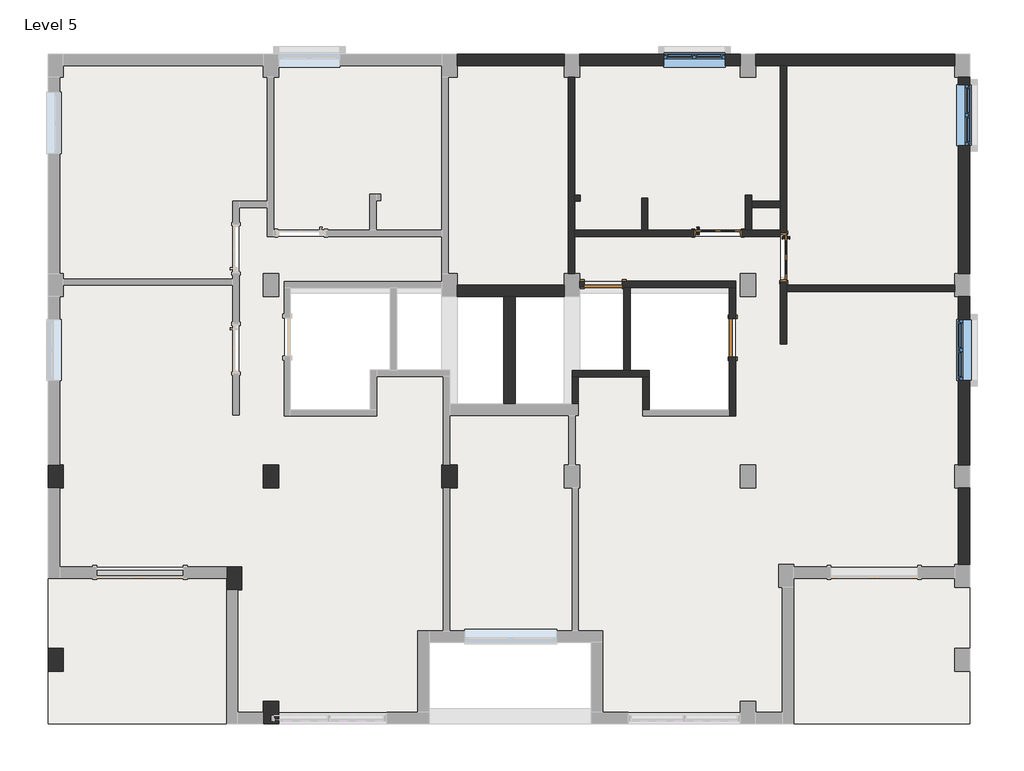
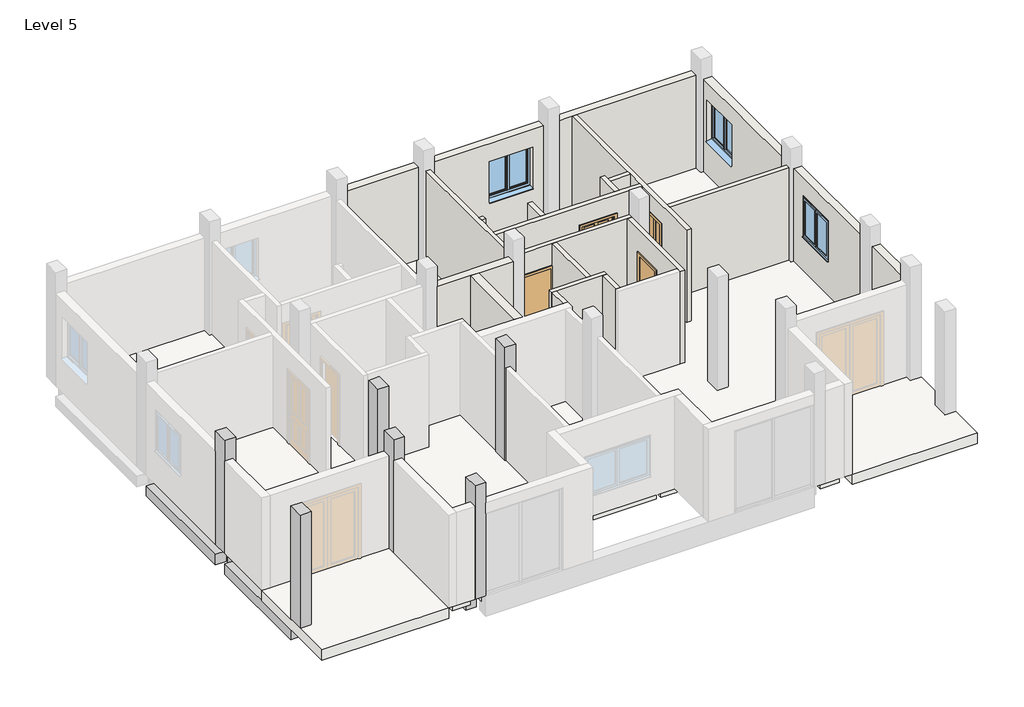
# One storey, part 2 of 3: 22 walls, 7 beams, 7 slabs, 6 columns, 4 doors, 3 windows.
"""IFC4 building model written with IfcOpenShell, lengths in millimetres."""

from ifc_helpers import new_model, si_unit, frame, origin, place, context, project, spatial, polyline, outline, extrude, faceted_brep, transform, mapped, element, save
from components import door_68a706ac, door_1fe7f57d, w2_0001_windows_4_x_4_9dec5fc7

model = new_model("IFC4")

# Units and contexts
model_context = context("Model", 3, world=origin())
ifc_project = project(units=[si_unit("LENGTHUNIT", "METRE", prefix="MILLI")], contexts=[model_context])

# Site, building, storey
site = spatial("IfcSite", under=ifc_project)
building = spatial("IfcBuilding", under=site)
storey = spatial("IfcBuildingStorey", under=building, Name="Level 5", Elevation=6400.8)

# Beams
placement = place(None, origin())
element("IfcBeam", 1, ObjectType="Concrete-Rectangular Beam : 12 x 24", at=placement, inside=storey, context=model_context, shape_type="SweptSolid", body=[
    extrude(outline(polyline([(-9144.7786397, -9410.6620333), (-9144.7786397, -6057.8620333), (-8839.9786397, -6057.8620333), (-8839.9786397, -9410.6620333), (-9144.7786397, -9410.6620333)])), frame((0.0, 0.0, 5791.2), z_axis=(0.0, 0.0, 1.0), x_axis=(1.0, 0.0, 0.0)), (0.0, 0.0, 1.0), 304.8),
])
element("IfcBeam", 2, ObjectType="Concrete-Rectangular Beam : 12 x 24", at=placement, inside=storey, context=model_context, shape_type="Brep", body=[
    faceted_brep([(-9144.7786397, -9867.8620333, 5791.2), (-9144.7786397, -13068.2620333, 5791.2), (-9144.7786397, -13068.2620333, 6096.0), (-9144.7786397, -9867.8620333, 6096.0), (-8839.9786397, -9867.8620333, 5791.2), (-8839.9786397, -11518.8620333, 5791.2), (-8839.9786397, -11823.6620333, 5791.2), (-8839.9786397, -13068.2620333, 5791.2), (-8839.9786397, -9867.8620333, 6096.0), (-8839.9786397, -11518.8620333, 6096.0), (-8839.9786397, -11823.6620333, 6096.0), (-8839.9786397, -13068.2620333, 6096.0)], [[[0, 1, 2, 3]], [[1, 0, 4, 5, 6, 7]], [[7, 6, 5, 4, 8, 9, 10, 11]], [[4, 0, 3, 8]], [[1, 7, 11, 2]], [[3, 2, 11, 10, 9, 8]]]),
])
element("IfcBeam", 3, ObjectType="Concrete-Rectangular Beam : 12 x 24", at=placement, inside=storey, context=model_context, shape_type="SweptSolid", body=[
    extrude(outline(polyline([(-4852.9175798, -9791.6620333), (-8839.9786397, -9791.6620333), (-8839.9786397, -9486.8620333), (-4852.9175798, -9486.8620333), (-4852.9175798, -9791.6620333)])), frame((0.0, 0.0, 5791.2), z_axis=(0.0, 0.0, 1.0), x_axis=(1.0, 0.0, 0.0)), (0.0, 0.0, 1.0), 304.8),
])
element("IfcBeam", 4, ObjectType="Concrete-Rectangular Beam : 12 x 24", at=placement, inside=storey, context=model_context, shape_type="SweptSolid", body=[
    extrude(outline(polyline([(-1296.9175798, -9791.6620333), (-4548.1175798, -9791.6620333), (-4548.1175798, -9486.8620333), (-1296.9175798, -9486.8620333), (-1296.9175798, -9791.6620333)])), frame((0.0, 0.0, 5791.2), z_axis=(0.0, 0.0, 1.0), x_axis=(1.0, 0.0, 0.0)), (0.0, 0.0, 1.0), 304.8),
])
element("IfcBeam", 5, ObjectType="Concrete-Rectangular Beam : 12 x 24", at=placement, inside=storey, context=model_context, shape_type="Brep", body=[
    faceted_brep([(-4852.9175798, -9867.8620333, 5791.2), (-4852.9175798, -11518.8620333, 5791.2), (-4852.9175798, -11823.6620333, 5791.2), (-4852.9175798, -14119.6402089, 5791.2), (-4852.9175798, -14119.6402089, 6096.0), (-4852.9175798, -11823.6620333, 6096.0), (-4852.9175798, -11518.8620333, 6096.0), (-4852.9175798, -9867.8620333, 6096.0), (-4548.1175798, -9867.8620333, 5791.2), (-4548.1175798, -14119.6402089, 5791.2), (-4548.1175798, -9867.8620333, 6096.0), (-4548.1175798, -14119.6402089, 6096.0)], [[[0, 1, 2, 3, 4, 5, 6, 7]], [[3, 2, 1, 0, 8, 9]], [[9, 8, 10, 11]], [[8, 0, 7, 10]], [[3, 9, 11, 4]], [[7, 6, 5, 4, 11, 10]]]),
])
element("IfcBeam", 6, ObjectType="Concrete-Rectangular Beam : 12 x 24", at=placement, inside=storey, context=model_context, shape_type="SweptSolid", body=[
    extrude(outline(polyline([(-4852.9175798, -11823.6620333), (-5284.7175798, -11823.6620333), (-5284.7175798, -11518.8620333), (-4852.9175798, -11518.8620333), (-4852.9175798, -11823.6620333)])), frame((0.0, 0.0, 5791.2), z_axis=(0.0, 0.0, 1.0), x_axis=(1.0, 0.0, 0.0)), (0.0, 0.0, 1.0), 304.8),
])
element("IfcBeam", 7, ObjectType="Concrete-Rectangular Beam : 12 x 24", at=placement, inside=storey, context=model_context, shape_type="SweptSolid", body=[
    extrude(outline(polyline([(-8839.9786397, -11518.8620333), (-5589.5175798, -11518.8620333), (-5589.5175798, -11823.6620333), (-8839.9786397, -11823.6620333), (-8839.9786397, -11518.8620333)])), frame((0.0, 0.0, 5791.2), z_axis=(0.0, 0.0, 1.0), x_axis=(1.0, 0.0, 0.0)), (0.0, 0.0, 1.0), 304.8),
])

# Columns
element("IfcColumn", 8, ObjectType="Concrete-Rectangular-Column : 1'6\" X 1' COLUMN", at=placement, inside=storey, context=model_context, shape_type="Brep", body=[
    faceted_brep([(-8839.9786397, -9410.6620333, 6400.8), (-8839.9786397, -9867.8620333, 6400.8), (-9144.7786397, -9867.8620333, 6400.8), (-9144.7786397, -9410.6620333, 6400.8), (-8839.9786397, -9410.6620333, 9753.6), (-8839.9786397, -9486.8620333, 9753.6), (-8839.9786397, -9791.6620333, 9753.6), (-8839.9786397, -9867.8620333, 9753.6), (-8839.9786397, -9867.8620333, 9144.0), (-8839.9786397, -9867.8620333, 8839.2), (-8839.9786397, -9867.8620333, 6705.6), (-8839.9786397, -9410.6620333, 6705.6), (-8839.9786397, -9410.6620333, 8839.2), (-8839.9786397, -9410.6620333, 9144.0), (-9144.7786397, -9867.8620333, 9753.6), (-9144.7786397, -9867.8620333, 9144.0), (-9144.7786397, -9867.8620333, 8839.2), (-9144.7786397, -9867.8620333, 6705.6), (-9144.7786397, -9410.6620333, 9753.6), (-9144.7786397, -9410.6620333, 9144.0), (-9144.7786397, -9410.6620333, 8839.2), (-9144.7786397, -9410.6620333, 6705.6)], [[[0, 1, 2, 3]], [[4, 5, 6, 7, 8, 9, 10, 1, 0, 11, 12, 13]], [[7, 14, 15, 16, 17, 2, 1, 10, 9, 8]], [[14, 18, 19, 20, 21, 3, 2, 17, 16, 15]], [[18, 4, 13, 12, 11, 0, 3, 21, 20, 19]], [[4, 18, 14, 7, 6, 5]]]),
])
element("IfcColumn", 9, ObjectType="Concrete-Rectangular-Column : 1'6\" X 1' COLUMN", at=placement, inside=storey, context=model_context, shape_type="Brep", body=[
    faceted_brep([(-4548.1175798, -9410.6620333, 6400.8), (-4548.1175798, -9867.8620333, 6400.8), (-4852.9175798, -9867.8620333, 6400.8), (-4852.9175798, -9410.6620333, 6400.8), (-4548.1175798, -9410.6620333, 9753.6), (-4548.1175798, -9486.8620333, 9753.6), (-4548.1175798, -9791.6620333, 9753.6), (-4548.1175798, -9867.8620333, 9753.6), (-4548.1175798, -9867.8620333, 9144.0), (-4548.1175798, -9867.8620333, 8839.2), (-4548.1175798, -9867.8620333, 6705.6), (-4548.1175798, -9410.6620333, 6705.6), (-4548.1175798, -9410.6620333, 8839.2), (-4548.1175798, -9410.6620333, 9144.0), (-4852.9175798, -9867.8620333, 9753.6), (-4852.9175798, -9867.8620333, 9144.0), (-4852.9175798, -9867.8620333, 8839.2), (-4852.9175798, -9867.8620333, 6705.6), (-4852.9175798, -9791.6620333, 9753.6), (-4852.9175798, -9486.8620333, 9753.6), (-4852.9175798, -9410.6620333, 9753.6), (-4852.9175798, -9410.6620333, 9144.0), (-4852.9175798, -9410.6620333, 8839.2), (-4852.9175798, -9410.6620333, 6705.6)], [[[0, 1, 2, 3]], [[4, 5, 6, 7, 8, 9, 10, 1, 0, 11, 12, 13]], [[7, 14, 15, 16, 17, 2, 1, 10, 9, 8]], [[14, 18, 19, 20, 21, 22, 23, 3, 2, 17, 16, 15]], [[20, 4, 13, 12, 11, 0, 3, 23, 22, 21]], [[4, 20, 19, 18, 14, 7, 6, 5]]]),
])
element("IfcColumn", 10, ObjectType="Concrete-Rectangular-Column : 1'6\" X 1' COLUMN", at=placement, inside=storey, context=model_context, shape_type="Brep", body=[
    faceted_brep([(-992.1175798, -9410.6620333, 6400.8), (-992.1175798, -9867.8620333, 6400.8), (-1296.9175798, -9867.8620333, 6400.8), (-1296.9175798, -9410.6620333, 6400.8), (-992.1175798, -9410.6620333, 9753.6), (-992.1175798, -9867.8620333, 9753.6), (-992.1175798, -9410.6620333, 6705.6), (-992.1175798, -9410.6620333, 8839.2), (-992.1175798, -9410.6620333, 9144.0), (-1296.9175798, -9867.8620333, 9753.6), (-1296.9175798, -9791.6620333, 9753.6), (-1296.9175798, -9486.8620333, 9753.6), (-1296.9175798, -9410.6620333, 9753.6), (-1296.9175798, -9410.6620333, 9144.0), (-1296.9175798, -9410.6620333, 8839.2), (-1296.9175798, -9410.6620333, 6705.6)], [[[0, 1, 2, 3]], [[4, 5, 1, 0, 6, 7, 8]], [[5, 9, 2, 1]], [[9, 10, 11, 12, 13, 14, 15, 3, 2]], [[12, 4, 8, 7, 6, 0, 3, 15, 14, 13]], [[4, 12, 11, 10, 9, 5]]]),
])
element("IfcColumn", 11, ObjectType="Concrete-Rectangular-Column : 1'6\" X 1' COLUMN", at=placement, inside=storey, context=model_context, shape_type="Brep", body=[
    faceted_brep([(-4548.1175798, -14119.6402089, 6400.8), (-4548.1175798, -14576.8402089, 6400.8), (-4852.9175798, -14576.8402089, 6400.8), (-4852.9175798, -14119.6402089, 6400.8), (-4548.1175798, -14119.6402089, 9753.6), (-4548.1175798, -14576.8402089, 9753.6), (-4548.1175798, -14576.8402089, 9448.8), (-4548.1175798, -14576.8402089, 8839.2), (-4548.1175798, -14119.6402089, 6705.6), (-4548.1175798, -14119.6402089, 8839.2), (-4548.1175798, -14119.6402089, 9144.0), (-4852.9175798, -14576.8402089, 9753.6), (-4852.9175798, -14119.6402089, 9753.6), (-4852.9175798, -14119.6402089, 9144.0), (-4852.9175798, -14119.6402089, 8839.2), (-4852.9175798, -14119.6402089, 6705.6)], [[[0, 1, 2, 3]], [[4, 5, 6, 7, 1, 0, 8, 9, 10]], [[5, 11, 2, 1, 7, 6]], [[11, 12, 13, 14, 15, 3, 2]], [[12, 4, 10, 9, 8, 0, 3, 15, 14, 13]], [[4, 12, 11, 5]]]),
])
element("IfcColumn", 12, ObjectType="Concrete-Rectangular-Column : 1'6\" X 1' COLUMN", at=placement, inside=storey, context=model_context, shape_type="Brep", body=[
    faceted_brep([(-8839.9786397, -13068.2620333, 6400.8), (-8839.9786397, -13525.4620333, 6400.8), (-9144.7786397, -13525.4620333, 6400.8), (-9144.7786397, -13068.2620333, 6400.8), (-8839.9786397, -13068.2620333, 9753.6), (-8839.9786397, -13525.4620333, 9753.6), (-8839.9786397, -13068.2620333, 6705.6), (-8839.9786397, -13068.2620333, 8839.2), (-8839.9786397, -13068.2620333, 9144.0), (-9144.7786397, -13525.4620333, 9753.6), (-9144.7786397, -13068.2620333, 9753.6), (-9144.7786397, -13068.2620333, 9144.0), (-9144.7786397, -13068.2620333, 8839.2), (-9144.7786397, -13068.2620333, 6705.6)], [[[0, 1, 2, 3]], [[4, 5, 1, 0, 6, 7, 8]], [[5, 9, 2, 1]], [[9, 10, 11, 12, 13, 3, 2]], [[10, 4, 8, 7, 6, 0, 3, 13, 12, 11]], [[4, 10, 9, 5]]]),
])
element("IfcColumn", 13, ObjectType="Concrete-Rectangular-Column : 1'6\" X 1' COLUMN", at=placement, inside=storey, context=model_context, shape_type="SweptSolid", body=[
    extrude(outline(polyline([(-5284.7175798, -11442.6620333), (-5284.7175798, -11899.8620333), (-5589.5175798, -11899.8620333), (-5589.5175798, -11442.6620333), (-5284.7175798, -11442.6620333)])), frame((0.0, 0.0, 6400.8), z_axis=(0.0, 0.0, 1.0), x_axis=(1.0, 0.0, 0.0)), (0.0, 0.0, 1.0), 3352.8),
])

# Doors
door_shape = door_68a706ac(model_context)
element("IfcDoor", 14, ObjectType="Door-Interior-Single-4_Panel-Wood : 36\" x 84\"", at=placement, inside=storey, context=model_context, shape_type="MappedRepresentation", body=[
    mapped(door_shape, transform((4202.1824202, -4789.1311634, 6400.8), x_axis=(1.0, 0.0, 0.0), y_axis=(0.0, 1.0, 0.0), z_axis=(0.0, 0.0, 1.0))),
])
element("IfcDoor", 15, ObjectType="Door-Interior-Single-4_Panel-Wood : 36\" x 84\"", at=placement, inside=storey, context=model_context, shape_type="MappedRepresentation", body=[
    mapped(door_shape, transform((5513.4574202, -5274.9061634, 6400.8), x_axis=(0.0, -1.0, 0.0), y_axis=(1.0, 0.0, 0.0), z_axis=(0.0, 0.0, 1.0))),
])
door_2_shape = door_1fe7f57d(model_context)
element("IfcDoor", 16, ObjectType="Single-Flush : 30\" x 80\"", at=placement, inside=storey, context=model_context, shape_type="MappedRepresentation", body=[
    mapped(door_2_shape, transform((1916.1824202, -5810.8691591, 6400.8), x_axis=(-1.0, 0.0, 0.0), y_axis=(0.0, -1.0, 0.0), z_axis=(0.0, 0.0, 1.0))),
])
element("IfcDoor", 17, ObjectType="Single-Flush : 30\" x 80\"", at=placement, inside=storey, context=model_context, shape_type="MappedRepresentation", body=[
    mapped(door_2_shape, transform((4494.2824202, -6877.6691591, 6400.8), x_axis=(0.0, 1.0, 0.0), y_axis=(-1.0, 0.0, 0.0), z_axis=(0.0, 0.0, 1.0))),
])

# Slabs
element("IfcSlab", 18, ObjectType="flooring 1'", at=placement, inside=storey, context=model_context, shape_type="SweptSolid", body=[
    extrude(outline(polyline([(-8916.1786397, -11442.6620333), (-8916.1786397, -9867.8620333), (-8839.9786397, -9867.8620333), (-8839.9786397, -9410.6620333), (-8916.1786397, -9410.6620333), (-8916.1786397, -6057.8620333), (-8839.9786397, -6057.8620333), (-8839.9786397, -5829.2620333), (-5462.5175798, -5829.2620333), (-5462.5175798, -8420.0620333), (-5335.5175798, -8420.0620333), (-5335.5175798, -4280.3104011), (-4776.7175798, -4280.3104011), (-4776.7175798, -4855.8061634), (-1296.9175798, -4855.8061634), (-1296.9175798, -5600.6620333), (-1296.9175798, -5758.8942903), (-4442.5950401, -5758.8942903), (-4442.5950401, -8439.1120333), (-2601.0950401, -8439.1120333), (-2601.0950401, -7651.7120333), (-1271.5175798, -7651.7120333), (-1271.5175798, -9410.6620333), (-1296.9175798, -9410.6620333), (-1296.9175798, -9867.8620333), (-1271.5175798, -9867.8620333), (-1271.5175798, -12722.6402089), (-1779.5175798, -12722.6402089), (-1779.5175798, -14348.2402089), (-4548.1175798, -14348.2402089), (-4548.1175798, -14119.6402089), (-4852.9175798, -14119.6402089), (-4852.9175798, -14348.2402089), (-5360.9175798, -14348.2402089), (-5360.9175798, -11899.8620333), (-5284.7175798, -11899.8620333), (-5284.7175798, -11442.6620333), (-5589.5175798, -11442.6620333), (-8916.1786397, -11442.6620333)])), frame((0.0, 0.0, 6096.0), z_axis=(0.0, 0.0, 1.0), x_axis=(1.0, 0.0, 0.0)), (0.0, 0.0, 1.0), 304.8),
])
element("IfcSlab", 19, ObjectType="flooring 1'", at=placement, inside=storey, context=model_context, shape_type="SweptSolid", body=[
    extrude(outline(polyline([(5446.7824202, -4855.8061634), (5446.7824202, -6583.0061634), (5573.7824202, -6583.0061634), (5573.7824202, -5956.2620333), (8913.8824202, -5956.2620333), (8913.8824202, -6057.8620333), (8990.0824202, -6057.8620333), (8990.0824202, -9410.6620333), (8913.8824202, -9410.6620333), (8913.8824202, -9867.8620333), (8990.0824202, -9867.8620333), (8990.0824202, -11391.8620333), (8913.8824202, -11391.8620333), (8913.8824202, -11442.6620333), (5713.4824202, -11442.6620333), (5713.4824202, -11391.8620333), (5408.6824202, -11391.8620333), (5408.6824202, -11849.0620333), (5484.8824202, -11849.0620333), (5484.8824202, -14348.2402089), (4951.4824202, -14348.2402089), (4951.4824202, -14119.6402089), (4646.6824202, -14119.6402089), (4646.6824202, -14348.2402089), (1903.4824202, -14348.2402089), (1903.4824202, -12722.6402089), (1420.8824202, -12722.6402089), (1420.8824202, -9867.8620333), (1446.2824202, -9867.8620333), (1446.2824202, -9410.6620333), (1357.3824202, -9410.6620333), (1357.3824202, -8426.4120333), (1420.8824202, -8426.4120333), (1420.8824202, -7660.8890971), (2703.5824202, -7660.8890971), (2703.5824202, -8439.7691591), (4557.7824202, -8439.7691591), (4557.7824202, -5747.3691591), (1446.2824202, -5747.3691591), (1446.2824202, -5600.6620333), (1344.6824202, -5600.6620333), (1344.6824202, -4855.8061634), (5446.7824202, -4855.8061634)])), frame((0.0, 0.0, 6096.0), z_axis=(0.0, 0.0, 1.0), x_axis=(1.0, 0.0, 0.0)), (0.0, 0.0, 1.0), 304.8),
])
element("IfcSlab", 20, ObjectType="flooring 1'", at=placement, inside=storey, context=model_context, shape_type="SweptSolid", body=[
    extrude(outline(polyline([(-8839.9786397, -1680.8061634), (-8839.9786397, -1452.2061634), (-4852.9175798, -1452.2061634), (-4852.9175798, -1680.8061634), (-4776.7175798, -1680.8061634), (-4776.7175798, -4153.3104011), (-5462.5175798, -4153.3104011), (-5462.5175798, -5702.2620333), (-8839.9786397, -5702.2620333), (-8839.9786397, -5600.6620333), (-8916.1786397, -5600.6620333), (-8916.1786397, -1680.8061634), (-8839.9786397, -1680.8061634)])), frame((0.0, 0.0, 6096.0), z_axis=(0.0, 0.0, 1.0), x_axis=(1.0, 0.0, 0.0)), (0.0, 0.0, 1.0), 304.8),
    extrude(outline(polyline([(-2732.0175798, -4728.8061634), (-4649.7175798, -4728.8061634), (-4649.7175798, -1680.8061634), (-4548.1175798, -1680.8061634), (-4548.1175798, -1452.2061634), (-1296.9175798, -1452.2061634), (-1296.9175798, -4728.8061634), (-2605.0175798, -4728.8061634), (-2605.0175798, -4144.6061634), (-2516.1175798, -4144.6061634), (-2516.1175798, -4017.6061634), (-2732.0175798, -4017.6061634), (-2732.0175798, -4728.8061634)])), frame((0.0, 0.0, 6096.0), z_axis=(0.0, 0.0, 1.0), x_axis=(1.0, 0.0, 0.0)), (0.0, 0.0, 1.0), 304.8),
])
element("IfcSlab", 21, ObjectType="flooring 1'", at=placement, inside=storey, context=model_context, shape_type="SweptSolid", body=[
    extrude(outline(polyline([(4646.6824202, -1452.2061634), (4646.6824202, -1680.8061634), (4951.4824202, -1680.8061634), (4951.4824202, -1452.2061634), (5446.7824202, -1452.2061634), (5446.7824202, -4157.3061634), (4875.2824202, -4157.3061634), (4875.2824202, -4030.3061634), (4748.2824202, -4030.3061634), (4748.2824202, -4728.8061634), (2805.1824202, -4728.8061634), (2805.1824202, -4093.8061634), (2678.1824202, -4093.8061634), (2678.1824202, -4728.8061634), (1344.6824202, -4728.8061634), (1344.6824202, -4157.3061634), (1458.9824202, -4157.3061634), (1458.9824202, -4030.3061634), (1344.6824202, -4030.3061634), (1344.6824202, -1680.8061634), (1446.2824202, -1680.8061634), (1446.2824202, -1452.2061634), (4646.6824202, -1452.2061634)])), frame((0.0, 0.0, 6096.0), z_axis=(0.0, 0.0, 1.0), x_axis=(1.0, 0.0, 0.0)), (0.0, 0.0, 1.0), 304.8),
    extrude(outline(polyline([(5446.7824202, -4284.3061634), (5446.7824202, -4728.8061634), (4875.2824202, -4728.8061634), (4875.2824202, -4284.3061634), (5446.7824202, -4284.3061634)])), frame((0.0, 0.0, 6096.0), z_axis=(0.0, 0.0, 1.0), x_axis=(1.0, 0.0, 0.0)), (0.0, 0.0, 1.0), 304.8),
    extrude(outline(polyline([(8913.8824202, -5829.2620333), (5573.7824202, -5829.2620333), (5573.7824202, -1452.2061634), (8913.8824202, -1452.2061634), (8913.8824202, -1680.8061634), (8990.0824202, -1680.8061634), (8990.0824202, -5600.6620333), (8913.8824202, -5600.6620333), (8913.8824202, -5829.2620333)])), frame((0.0, 0.0, 6096.0), z_axis=(0.0, 0.0, 1.0), x_axis=(1.0, 0.0, 0.0)), (0.0, 0.0, 1.0), 304.8),
])
element("IfcSlab", 22, ObjectType="flooring 1'", at=placement, inside=storey, context=model_context, shape_type="SweptSolid", body=[
    extrude(outline(polyline([(1141.4824202, -1452.2061634), (1141.4824202, -1680.8061634), (1217.6824202, -1680.8061634), (1217.6824202, -5600.6620333), (1141.4824202, -5600.6620333), (1141.4824202, -5829.2620333), (-992.1175798, -5829.2620333), (-992.1175798, -5600.6620333), (-1169.9175798, -5600.6620333), (-1169.9175798, -1680.8061634), (-992.1175798, -1680.8061634), (-992.1175798, -1452.2061634), (1141.4824202, -1452.2061634)])), frame((0.0, 0.0, 6096.0), z_axis=(0.0, 0.0, 1.0), x_axis=(1.0, 0.0, 0.0)), (0.0, 0.0, 1.0), 304.8),
])
element("IfcSlab", 23, ObjectType="flooring 1'", at=placement, inside=storey, context=model_context, shape_type="SweptSolid", body=[
    extrude(outline(polyline([(1293.8824202, -12722.6402089), (-1144.5175798, -12722.6402089), (-1144.5175798, -9867.8620333), (-992.1175798, -9867.8620333), (-992.1175798, -9410.6620333), (-1144.5175798, -9410.6620333), (-1144.5175798, -8426.4120333), (1230.3824202, -8426.4120333), (1230.3824202, -9410.6620333), (1141.4824202, -9410.6620333), (1141.4824202, -9867.8620333), (1293.8824202, -9867.8620333), (1293.8824202, -12722.6402089)])), frame((0.0, 0.0, 6096.0), z_axis=(0.0, 0.0, 1.0), x_axis=(1.0, 0.0, 0.0)), (0.0, 0.0, 1.0), 304.8),
])
element("IfcSlab", 24, ObjectType="flooring 1'", at=placement, inside=storey, context=model_context, shape_type="SweptSolid", body=[
    extrude(outline(polyline([(-5589.5175798, -11671.2620333), (-5589.5175798, -14576.8402089), (-9144.7786397, -14576.8402089), (-9144.7786397, -11671.2620333), (-5589.5175798, -11671.2620333)])), frame((0.0, 0.0, 6096.0), z_axis=(0.0, 0.0, 1.0), x_axis=(1.0, 0.0, 0.0)), (0.0, 0.0, 1.0), 304.8),
    extrude(outline(polyline([(9218.6824202, -11671.2620333), (9218.6824202, -14576.8402089), (5713.4824202, -14576.8402089), (5713.4824202, -11671.2620333), (9218.6824202, -11671.2620333)])), frame((0.0, 0.0, 6096.0), z_axis=(0.0, 0.0, 1.0), x_axis=(1.0, 0.0, 0.0)), (0.0, 0.0, 1.0), 304.8),
])

# Walls
element("IfcWall", 25, ObjectType="EXTERIOR WALL 9\"", at=placement, inside=storey, context=model_context, shape_type="SweptSolid", body=[
    extrude(outline(polyline([(1141.4824202, -1452.2061634), (-992.1175798, -1452.2061634), (-992.1175798, -1223.6061634), (1141.4824202, -1223.6061634), (1141.4824202, -1452.2061634)])), frame((0.0, 0.0, 6400.8), z_axis=(0.0, 0.0, 1.0), x_axis=(1.0, 0.0, 0.0)), (0.0, 0.0, 1.0), 2743.2),
])
element("IfcWall", 26, ObjectType="EXTERIOR WALL 9\"", at=placement, inside=storey, context=model_context, shape_type="SweptSolid", body=[
    extrude(outline(polyline([(6400.8, 1446.2824202), (6400.8, 4646.6824202), (9144.0, 4646.6824202), (9144.0, 1446.2824202), (6400.8, 1446.2824202)]), holes=[polyline([(7400.8, 4341.8824202), (7400.8, 3122.6824202), (8620.0, 3122.6824202), (8620.0, 4341.8824202), (7400.8, 4341.8824202)])]), frame((0.0, -1452.2061634, 0.0), z_axis=(0.0, 1.0, 0.0), x_axis=(0.0, 0.0, 1.0)), (0.0, 0.0, 1.0), 228.6),
])
element("IfcWall", 27, ObjectType="EXTERIOR WALL 9\"", at=placement, inside=storey, context=model_context, shape_type="Brep", body=[
    faceted_brep([(4951.4824202, -1452.2061634, 6400.8), (5446.7824202, -1452.2061634, 6400.8), (5573.7824202, -1452.2061634, 6400.8), (8913.8824202, -1452.2061634, 6400.8), (8913.8824202, -1452.2061634, 9144.0), (5573.7824202, -1452.2061634, 9144.0), (5446.7824202, -1452.2061634, 9144.0), (4951.4824202, -1452.2061634, 9144.0), (4951.4824202, -1223.6061634, 6400.8), (4951.4824202, -1223.6061634, 9144.0), (8913.8824202, -1223.6061634, 9144.0), (8913.8824202, -1223.6061634, 6400.8)], [[[0, 1, 2, 3, 4, 5, 6, 7]], [[8, 9, 10, 11]], [[3, 2, 1, 0, 8, 11]], [[4, 3, 11, 10]], [[7, 6, 5, 4, 10, 9]], [[0, 7, 9, 8]]]),
])
element("IfcWall", 28, ObjectType="EXTERIOR WALL 9\"", at=placement, inside=storey, context=model_context, shape_type="SweptSolid", body=[
    extrude(outline(polyline([(-1680.8061634, 6400.8), (-5600.6620333, 6400.8), (-5600.6620333, 9144.0), (-1680.8061634, 9144.0), (-1680.8061634, 6400.8)]), holes=[polyline([(-3052.4061634, 7400.8), (-1833.2061634, 7400.8), (-1833.2061634, 8620.0), (-3052.4061634, 8620.0), (-3052.4061634, 7400.8)])]), frame((8990.0824202, 0.0, 0.0), z_axis=(1.0, 0.0, 0.0), x_axis=(0.0, 1.0, 0.0)), (0.0, 0.0, 1.0), 228.6),
])
element("IfcWall", 29, ObjectType="EXTERIOR WALL 9\"", at=placement, inside=storey, context=model_context, shape_type="SweptSolid", body=[
    extrude(outline(polyline([(-6057.8620333, 6400.8), (-9410.6620333, 6400.8), (-9410.6620333, 9144.0), (-6057.8620333, 9144.0), (-6057.8620333, 6400.8)]), holes=[polyline([(-6515.0620333, 7400.8), (-6515.0620333, 8620.0), (-7734.2620333, 8620.0), (-7734.2620333, 7400.8), (-6515.0620333, 7400.8)])]), frame((8990.0824202, 0.0, 0.0), z_axis=(1.0, 0.0, 0.0), x_axis=(0.0, 1.0, 0.0)), (0.0, 0.0, 1.0), 228.6),
])
element("IfcWall", 30, ObjectType="EXTERIOR WALL 9\"", at=placement, inside=storey, context=model_context, shape_type="SweptSolid", body=[
    extrude(outline(polyline([(8990.0824202, -11391.8620333), (8990.0824202, -9867.8620333), (9218.6824202, -9867.8620333), (9218.6824202, -11391.8620333), (8990.0824202, -11391.8620333)])), frame((0.0, 0.0, 6400.8), z_axis=(0.0, 0.0, 1.0), x_axis=(1.0, 0.0, 0.0)), (0.0, 0.0, 1.0), 2743.2),
])
element("IfcWall", 31, ObjectType="EXTERIOR WALL 9\"", at=placement, inside=storey, context=model_context, shape_type="Brep", body=[
    faceted_brep([(1141.4824202, -5829.2620333, 6400.8), (-992.1175798, -5829.2620333, 6400.8), (-992.1175798, -5829.2620333, 9144.0), (1141.4824202, -5829.2620333, 9144.0), (1141.4824202, -6057.8620333, 6400.8), (1141.4824202, -6057.8620333, 9144.0), (163.5824202, -6057.8620333, 9144.0), (-65.0175798, -6057.8620333, 9144.0), (-992.1175798, -6057.8620333, 9144.0), (-992.1175798, -6057.8620333, 6400.8), (-65.0175798, -6057.8620333, 6400.8), (163.5824202, -6057.8620333, 6400.8)], [[[0, 1, 2, 3]], [[4, 5, 6, 7, 8, 9, 10, 11]], [[1, 0, 4, 11, 10, 9]], [[2, 1, 9, 8]], [[3, 2, 8, 7, 6, 5]], [[0, 3, 5, 4]]]),
])
element("IfcWall", 32, ObjectType="EXTERIOR WALL 9\"", at=placement, inside=storey, context=model_context, shape_type="SweptSolid", body=[
    extrude(outline(polyline([(-65.0175798, -8197.8120333), (-65.0175798, -6057.8620333), (163.5824202, -6057.8620333), (163.5824202, -8197.8120333), (-65.0175798, -8197.8120333)])), frame((0.0, 0.0, 6400.8), z_axis=(0.0, 0.0, 1.0), x_axis=(1.0, 0.0, 0.0)), (0.0, 0.0, 1.0), 2743.2),
])
element("IfcWall", 33, ObjectType="INTERIOR WALL 5\"", at=placement, inside=storey, context=model_context, shape_type="Brep", body=[
    faceted_brep([(1217.6824202, -1680.8061634, 6400.8), (1217.6824202, -5600.6620333, 6400.8), (1217.6824202, -5600.6620333, 9144.0), (1217.6824202, -1680.8061634, 9144.0), (1344.6824202, -1680.8061634, 6400.8), (1344.6824202, -1680.8061634, 9144.0), (1344.6824202, -4030.3061634, 9144.0), (1344.6824202, -4157.3061634, 9144.0), (1344.6824202, -4728.8061634, 9144.0), (1344.6824202, -4855.8061634, 9144.0), (1344.6824202, -5600.6620333, 9144.0), (1344.6824202, -5600.6620333, 6400.8), (1344.6824202, -4855.8061634, 6400.8), (1344.6824202, -4728.8061634, 6400.8), (1344.6824202, -4157.3061634, 6400.8), (1344.6824202, -4030.3061634, 6400.8)], [[[0, 1, 2, 3]], [[4, 5, 6, 7, 8, 9, 10, 11, 12, 13, 14, 15]], [[1, 0, 4, 15, 14, 13, 12, 11]], [[2, 1, 11, 10]], [[3, 2, 10, 9, 8, 7, 6, 5]], [[0, 3, 5, 4]]]),
])
element("IfcWall", 34, ObjectType="INTERIOR WALL 5\"", at=placement, inside=storey, context=model_context, shape_type="Brep", body=[
    faceted_brep([(5446.7824202, -4855.8061634, 9144.0), (1344.6824202, -4855.8061634, 9144.0), (1344.6824202, -4855.8061634, 6400.8), (3719.5824202, -4855.8061634, 6400.8), (3719.5824202, -4855.8061634, 8559.8), (4684.7824202, -4855.8061634, 8559.8), (4684.7824202, -4855.8061634, 6400.8), (5446.7824202, -4855.8061634, 6400.8), (1344.6824202, -4728.8061634, 9144.0), (2678.1824202, -4728.8061634, 9144.0), (2805.1824202, -4728.8061634, 9144.0), (4748.2824202, -4728.8061634, 9144.0), (4875.2824202, -4728.8061634, 9144.0), (5446.7824202, -4728.8061634, 9144.0), (5446.7824202, -4728.8061634, 6400.8), (4875.2824202, -4728.8061634, 6400.8), (4748.2824202, -4728.8061634, 6400.8), (4684.7824202, -4728.8061634, 6400.8), (4684.7824202, -4728.8061634, 8559.8), (3719.5824202, -4728.8061634, 8559.8), (3719.5824202, -4728.8061634, 6400.8), (2805.1824202, -4728.8061634, 6400.8), (2678.1824202, -4728.8061634, 6400.8), (1344.6824202, -4728.8061634, 6400.8)], [[[0, 1, 2, 3, 4, 5, 6, 7]], [[8, 9, 10, 11, 12, 13, 14, 15, 16, 17, 18, 19, 20, 21, 22, 23]], [[2, 23, 22, 21, 20, 3]], [[14, 7, 6, 17, 16, 15]], [[1, 0, 13, 12, 11, 10, 9, 8]], [[2, 1, 8, 23]], [[0, 7, 14, 13]], [[5, 18, 17, 6]], [[18, 5, 4, 19]], [[19, 4, 3, 20]]]),
])
element("IfcWall", 35, ObjectType="INTERIOR WALL 5\"", at=placement, inside=storey, context=model_context, shape_type="Brep", body=[
    faceted_brep([(4875.2824202, -4728.8061634, 6400.8), (4875.2824202, -4284.3061634, 6400.8), (4875.2824202, -4157.3061634, 6400.8), (4875.2824202, -4030.3061634, 6400.8), (4875.2824202, -4030.3061634, 9144.0), (4875.2824202, -4157.3061634, 9144.0), (4875.2824202, -4284.3061634, 9144.0), (4875.2824202, -4728.8061634, 9144.0), (4748.2824202, -4728.8061634, 6400.8), (4748.2824202, -4728.8061634, 9144.0), (4748.2824202, -4030.3061634, 9144.0), (4748.2824202, -4030.3061634, 6400.8)], [[[0, 1, 2, 3, 4, 5, 6, 7]], [[8, 9, 10, 11]], [[3, 2, 1, 0, 8, 11]], [[4, 3, 11, 10]], [[7, 6, 5, 4, 10, 9]], [[0, 7, 9, 8]]]),
])
element("IfcWall", 36, ObjectType="INTERIOR WALL 5\"", at=placement, inside=storey, context=model_context, shape_type="SweptSolid", body=[
    extrude(outline(polyline([(5446.7824202, -4284.3061634), (4875.2824202, -4284.3061634), (4875.2824202, -4157.3061634), (5446.7824202, -4157.3061634), (5446.7824202, -4284.3061634)])), frame((0.0, 0.0, 6400.8), z_axis=(0.0, 0.0, 1.0), x_axis=(1.0, 0.0, 0.0)), (0.0, 0.0, 1.0), 2743.2),
])
element("IfcWall", 37, ObjectType="INTERIOR WALL 5\"", at=placement, inside=storey, context=model_context, shape_type="Brep", body=[
    faceted_brep([(5446.7824202, -7002.1061634, 6400.8), (5446.7824202, -7002.1061634, 9144.0), (5446.7824202, -4855.8061634, 9144.0), (5446.7824202, -4728.8061634, 9144.0), (5446.7824202, -4284.3061634, 9144.0), (5446.7824202, -4157.3061634, 9144.0), (5446.7824202, -1452.2061634, 9144.0), (5446.7824202, -1452.2061634, 6400.8), (5446.7824202, -4157.3061634, 6400.8), (5446.7824202, -4284.3061634, 6400.8), (5446.7824202, -4728.8061634, 6400.8), (5446.7824202, -4792.3061634, 6400.8), (5446.7824202, -4792.3061634, 8559.8), (5446.7824202, -5757.5061634, 8559.8), (5446.7824202, -5757.5061634, 6400.8), (5573.7824202, -7002.1061634, 9144.0), (5573.7824202, -7002.1061634, 6400.8), (5573.7824202, -5956.2620333, 6400.8), (5573.7824202, -5829.2620333, 6400.8), (5573.7824202, -5757.5061634, 6400.8), (5573.7824202, -5757.5061634, 8559.8), (5573.7824202, -4792.3061634, 8559.8), (5573.7824202, -4792.3061634, 6400.8), (5573.7824202, -1452.2061634, 6400.8), (5573.7824202, -1452.2061634, 9144.0), (5573.7824202, -5829.2620333, 9144.0), (5573.7824202, -5956.2620333, 9144.0)], [[[0, 1, 2, 3, 4, 5, 6, 7, 8, 9, 10, 11, 12, 13, 14]], [[15, 16, 17, 18, 19, 20, 21, 22, 23, 24, 25, 26]], [[16, 0, 14, 19, 18, 17]], [[7, 23, 22, 11, 10, 9, 8]], [[1, 0, 16, 15]], [[6, 5, 4, 3, 2, 1, 15, 26, 25, 24]], [[7, 6, 24, 23]], [[13, 20, 19, 14]], [[20, 13, 12, 21]], [[21, 12, 11, 22]]]),
])
element("IfcWall", 38, ObjectType="INTERIOR WALL 5\"", at=placement, inside=storey, context=model_context, shape_type="SweptSolid", body=[
    extrude(outline(polyline([(5573.7824202, -5829.2620333), (8913.8824202, -5829.2620333), (8913.8824202, -5956.2620333), (5573.7824202, -5956.2620333), (5573.7824202, -5829.2620333)])), frame((0.0, 0.0, 6400.8), z_axis=(0.0, 0.0, 1.0), x_axis=(1.0, 0.0, 0.0)), (0.0, 0.0, 1.0), 2743.2),
])
element("IfcWall", 39, ObjectType="INTERIOR WALL 5\"", at=placement, inside=storey, context=model_context, shape_type="SweptSolid", body=[
    extrude(outline(polyline([(2805.1824202, -4093.8061634), (2805.1824202, -4728.8061634), (2678.1824202, -4728.8061634), (2678.1824202, -4093.8061634), (2805.1824202, -4093.8061634)])), frame((0.0, 0.0, 6400.8), z_axis=(0.0, 0.0, 1.0), x_axis=(1.0, 0.0, 0.0)), (0.0, 0.0, 1.0), 2743.2),
])
element("IfcWall", 40, ObjectType="INTERIOR WALL 5\"", at=placement, inside=storey, context=model_context, shape_type="SweptSolid", body=[
    extrude(outline(polyline([(1458.9824202, -4157.3061634), (1344.6824202, -4157.3061634), (1344.6824202, -4030.3061634), (1458.9824202, -4030.3061634), (1458.9824202, -4157.3061634)])), frame((0.0, 0.0, 6400.8), z_axis=(0.0, 0.0, 1.0), x_axis=(1.0, 0.0, 0.0)), (0.0, 0.0, 1.0), 2743.2),
])
element("IfcWall", 41, ObjectType="INTERIOR WALL 5\"", at=placement, inside=storey, context=model_context, shape_type="Brep", body=[
    faceted_brep([(1535.1824202, -5747.3691591, 8432.8), (1535.1824202, -5747.3691591, 6400.8), (1446.2824202, -5747.3691591, 6400.8), (1446.2824202, -5747.3691591, 9144.0), (4557.7824202, -5747.3691591, 9144.0), (4557.7824202, -5747.3691591, 6400.8), (2297.1824202, -5747.3691591, 6400.8), (2297.1824202, -5747.3691591, 8432.8), (1446.2824202, -5874.3691591, 6400.8), (1535.1824202, -5874.3691591, 6400.8), (1535.1824202, -5874.3691591, 8432.8), (2297.1824202, -5874.3691591, 8432.8), (2297.1824202, -5874.3691591, 6400.8), (2322.5824202, -5874.3691591, 6400.8), (2449.5824202, -5874.3691591, 6400.8), (4430.7824202, -5874.3691591, 6400.8), (4557.7824202, -5874.3691591, 6400.8), (4557.7824202, -5874.3691591, 9144.0), (4430.7824202, -5874.3691591, 9144.0), (2449.5824202, -5874.3691591, 9144.0), (2322.5824202, -5874.3691591, 9144.0), (1446.2824202, -5874.3691591, 9144.0)], [[[0, 1, 2, 3, 4, 5, 6, 7]], [[8, 9, 10, 11, 12, 13, 14, 15, 16, 17, 18, 19, 20, 21]], [[6, 5, 16, 15, 14, 13, 12]], [[2, 1, 9, 8]], [[3, 2, 8, 21]], [[4, 3, 21, 20, 19, 18, 17]], [[5, 4, 17, 16]], [[10, 9, 1, 0]], [[11, 10, 0, 7]], [[12, 11, 7, 6]]]),
])
element("IfcWall", 42, ObjectType="INTERIOR WALL 5\"", at=placement, inside=storey, context=model_context, shape_type="Brep", body=[
    faceted_brep([(4430.7824202, -5874.3691591, 6400.8), (4430.7824202, -6496.6691591, 6400.8), (4430.7824202, -6496.6691591, 8432.8), (4430.7824202, -7258.6691591, 8432.8), (4430.7824202, -7258.6691591, 6400.8), (4430.7824202, -8312.7691591, 6400.8), (4430.7824202, -8439.7691591, 6400.8), (4430.7824202, -8439.7691591, 9144.0), (4430.7824202, -8312.7691591, 9144.0), (4430.7824202, -5874.3691591, 9144.0), (4557.7824202, -6496.6691591, 8432.8), (4557.7824202, -6496.6691591, 6400.8), (4557.7824202, -5874.3691591, 6400.8), (4557.7824202, -5874.3691591, 9144.0), (4557.7824202, -8439.7691591, 9144.0), (4557.7824202, -8439.7691591, 6400.8), (4557.7824202, -7258.6691591, 6400.8), (4557.7824202, -7258.6691591, 8432.8)], [[[0, 1, 2, 3, 4, 5, 6, 7, 8, 9]], [[10, 11, 12, 13, 14, 15, 16, 17]], [[16, 15, 6, 5, 4]], [[12, 11, 1, 0]], [[9, 8, 7, 14, 13]], [[0, 9, 13, 12]], [[7, 6, 15, 14]], [[2, 1, 11, 10]], [[3, 2, 10, 17]], [[4, 3, 17, 16]]]),
])
element("IfcWall", 43, ObjectType="INTERIOR WALL 5\"", at=placement, inside=storey, context=model_context, shape_type="SweptSolid", body=[
    extrude(outline(polyline([(2830.5824202, -7660.8890971), (2830.5824202, -8312.7691591), (2703.5824202, -8312.7691591), (2703.5824202, -7660.8890971), (2830.5824202, -7660.8890971)])), frame((0.0, 0.0, 6400.8), z_axis=(0.0, 0.0, 1.0), x_axis=(1.0, 0.0, 0.0)), (0.0, 0.0, 1.0), 2743.2),
])
element("IfcWall", 44, ObjectType="INTERIOR WALL 5\"", at=placement, inside=storey, context=model_context, shape_type="Brep", body=[
    faceted_brep([(2830.5824202, -7533.8890971, 6400.8), (2449.5824202, -7533.8890971, 6400.8), (2322.5824202, -7533.8890971, 6400.8), (1293.8824202, -7533.8890971, 6400.8), (1293.8824202, -7533.8890971, 9144.0), (2322.5824202, -7533.8890971, 9144.0), (2449.5824202, -7533.8890971, 9144.0), (2830.5824202, -7533.8890971, 9144.0), (2830.5824202, -7660.8890971, 6400.8), (2830.5824202, -7660.8890971, 9144.0), (2703.5824202, -7660.8890971, 9144.0), (1420.8824202, -7660.8890971, 9144.0), (1293.8824202, -7660.8890971, 9144.0), (1293.8824202, -7660.8890971, 6400.8), (1420.8824202, -7660.8890971, 6400.8), (2703.5824202, -7660.8890971, 6400.8)], [[[0, 1, 2, 3, 4, 5, 6, 7]], [[8, 9, 10, 11, 12, 13, 14, 15]], [[3, 2, 1, 0, 8, 15, 14, 13]], [[7, 6, 5, 4, 12, 11, 10, 9]], [[0, 7, 9, 8]], [[4, 3, 13, 12]]]),
])
element("IfcWall", 45, ObjectType="INTERIOR WALL 5\"", at=placement, inside=storey, context=model_context, shape_type="SweptSolid", body=[
    extrude(outline(polyline([(1293.8824202, -8197.8120333), (1293.8824202, -7660.8890971), (1420.8824202, -7660.8890971), (1420.8824202, -8197.8120333), (1293.8824202, -8197.8120333)])), frame((0.0, 0.0, 6400.8), z_axis=(0.0, 0.0, 1.0), x_axis=(1.0, 0.0, 0.0)), (0.0, 0.0, 1.0), 2743.2),
])
element("IfcWall", 46, ObjectType="INTERIOR WALL 5\"", at=placement, inside=storey, context=model_context, shape_type="SweptSolid", body=[
    extrude(outline(polyline([(2322.5824202, -7533.8890971), (2322.5824202, -5874.3691591), (2449.5824202, -5874.3691591), (2449.5824202, -7533.8890971), (2322.5824202, -7533.8890971)])), frame((0.0, 0.0, 6400.8), z_axis=(0.0, 0.0, 1.0), x_axis=(1.0, 0.0, 0.0)), (0.0, 0.0, 1.0), 2743.2),
])

# Windows
w2_0001_windows_4_x_4_shape = w2_0001_windows_4_x_4_9dec5fc7(model_context)
element("IfcWindow", 47, ObjectType="w2.0001 : WINDOWS 4' X 4'", at=placement, inside=storey, context=model_context, shape_type="MappedRepresentation", body=[
    mapped(w2_0001_windows_4_x_4_shape, transform((9104.3824202, -7124.6620333, 6400.8), x_axis=(0.0, -1.0, 0.0), y_axis=(1.0, 0.0, 0.0), z_axis=(0.0, 0.0, 1.0))),
])
element("IfcWindow", 48, ObjectType="w2.0001 : WINDOWS 4' X 4'", at=placement, inside=storey, context=model_context, shape_type="MappedRepresentation", body=[
    mapped(w2_0001_windows_4_x_4_shape, transform((9104.3824202, -2442.8061634, 6400.8), x_axis=(0.0, 1.0, 0.0), y_axis=(-1.0, 0.0, 0.0), z_axis=(0.0, 0.0, 1.0))),
])
element("IfcWindow", 49, ObjectType="w2.0001 : WINDOWS 4' X 4'", at=placement, inside=storey, context=model_context, shape_type="MappedRepresentation", body=[
    mapped(w2_0001_windows_4_x_4_shape, transform((3732.2824202, -1337.9061634, 6400.8), x_axis=(-1.0, 0.0, 0.0), y_axis=(0.0, -1.0, 0.0), z_axis=(0.0, 0.0, 1.0))),
])

save(model, "model.ifc")

# Revit data of these elements
# Type "Concrete-Rectangular Beam : 12 x 24"
#   Assembly Code = "B10"
#   Length [instance default] = 5' - 0"
#   b = 1' - 0"
#   h = 2' - 0"
#   Structural Material [instance default] = Concrete, Cast-in-Place gray
# Type "Concrete-Rectangular-Column : 1'6\" X 1' COLUMN"
#   Assembly Code = "B10"
#   b = 1' - 0"
#   h = 1' - 6"
#   Structural Material [instance default] = Concrete, Cast-in-Place gray
# Type "Door-Interior-Single-4_Panel-Wood : 36\" x 84\""
#   Type Mark = "9"
#   Assembly Code = "C1020300"
#   Analytic Construction = "Wooden"
#   Top Rail = 0' - 4 11/16"
#   Thickness = 0' - 1 3/8"
#   Thermal Resistance (R) = 2.5876 (h·ft²·°F)/BTU
#   Swing Angle [instance default] = 90.00°
#   Stiles = 0' - 4 3/4"
#   Rough Width = 3' - 2"
#   Rough Height = 7' - 1"
#   Mullion = 0' - 4 1/2"
#   Lock Rail = 0' - 7 1/2"
#   Height = 7' - 0"
#   Width = 3' - 0"
#   Heat Transfer Coefficient (U) = 0.3865 BTU/(h·ft²·°F)
#   Bottom Rail = 0' - 9 1/8"
#   Trim Material = Cherry
#   Panel Material = Cherry
#   Frame Material = Cherry
#   Door Handle Material = Aluminum
#   Visual Light Transmittance = 0
#   Solar Heat Gain Coefficient = 0
#   Wall Closure = (empty or 0)
#   Function = (empty or 0)
# Type "Single-Flush : 30\" x 80\""
#   Type Mark = "5"
#   Construction Type Id = "MDOOR"
#   Assembly Code = "C1020"
#   Analytic Construction = "Metal"
#   Thickness = 0' - 2"
#   Heat Transfer Coefficient (U) = 0.651978 BTU/(h·ft²·°F)
#   Height = 6' - 8"
#   Trim Projection Ext = 0' - 1"
#   Trim Projection Int = 0' - 1"
#   Trim Width = 0' - 3"
#   Width = 2' - 6"
#   Define Thermal Properties by = 1
#   Define Thermal Properties by = 1
#   Door Material = Door - Panel
#   Frame Material = Door - Frame
#   Visual Light Transmittance = 0
#   Solar Heat Gain Coefficient = 0
#   Function = (empty or 0)
#   Wall Closure = (empty or 0)
# Type "flooring 1'"
#   Assembly Code = "B1010"
#   Function = 0
#   Layers, outside or top first: 1' - 0" "FL_MARBLE WHITE" (function 1)
# Type "EXTERIOR WALL 9\""
#   Assembly Code = "B2010"
#   Layers, outside or top first: 0' - 9" "WARM BEIGE COLOUR" (function 1)
# Type "INTERIOR WALL 5\""
#   Assembly Code = "B2010"
#   Layers, outside or top first: 0' - 5" "WARM BEIGE COLOUR" (function 1)
# Type "w2.0001 : WINDOWS 4' X 4'"
#   Type Mark = "21"
#   Operation = "DoublePanelVertical"
#   Keynote = "16.05.01"
#   Analytic Construction = "<None>"
#   Rough Width = 4' - 0"
#   Rough Height = 4' - 0"
#   Rahmentiefe = 0' - 2.3622"
#   Rahmenhöhe unten = 0' - 3.14961"
#   Rahmehöhe oben = 0' - 3.14961"
#   Rahmenbreite = 0' - 2.3622"
#   Height = 4' - 0"
#   Flügeltiefe = 0' - 2.3622"
#   Flügelbreite = 0' - 2.3622"
#   Einbautiefe (von außen) [instance default] = 0' - 5.51181"
#   Width = 4' - 0"
#   Kippflügel [instance default] = yes
#   Drehflügel im Grundriß darstellen [instance default] = no
#   Drehflügel [instance default] = yes
#   Define Thermal Properties by = 1
#   Rahmen [instance default] = none
#   Glas [instance default] = none
#   Flügel [instance default] = none
#   Fensterbank aussen [instance default] = none
#   Fensterbank innen [instance default] = none
#   Wall Closure = (empty or 0)
# Elements 1, 2, 3, 4, 5, 6, 7 (IfcBeam, "Concrete-Rectangular Beam : 12 x 24")
#   Structural Material = WARM BEIGE COLOUR
#   Phase Created = New Construction
#   Materials on its faces: "WARM BEIGE COLOUR"
# Elements 8, 9, 10, 11, 12, 13 (IfcColumn, "Concrete-Rectangular-Column : 1'6\" X 1' COLUMN")
#   Structural Material = WARM BEIGE COLOUR
#   Phase Created = New Construction
#   Materials on its faces: "WARM BEIGE COLOUR"
# Elements 14, 15 (IfcDoor, "Door-Interior-Single-4_Panel-Wood : 36\" x 84\"")
#   Swing Angle = 90.00°
#   Phase Created = New Construction
#   Materials on its faces: "Cherry", "Aluminum"
# Elements 16, 17 (IfcDoor, "Single-Flush : 30\" x 80\"")
#   Phase Created = New Construction
#   Materials on its faces: "Door - Frame", "Door - Panel"
# Element 18 (IfcSlab, "flooring 1'")
#   built-in parameter 1001955 = 3.14159 (stored number, unit not read)
#   Height Offset From Level = 0' - 0"
#   Phase Created = New Construction
#   Materials on its faces: "FL_MARBLE WHITE"
# Elements 19, 21, 22, 23, 24 (IfcSlab, "flooring 1'")
#   Height Offset From Level = 0' - 0"
#   Phase Created = New Construction
#   Materials on its faces: "FL_MARBLE WHITE"
# Element 20 (IfcSlab, "flooring 1'")
#   built-in parameter 1001955 = -1.5708 (stored number, unit not read)
#   Height Offset From Level = 0' - 0"
#   Phase Created = New Construction
#   Materials on its faces: "FL_MARBLE WHITE"
# Elements 25, 26, 27, 28, 29, 30, 31, 32 (IfcWall, "EXTERIOR WALL 9\"")
#   Top Offset = -1' - 0"
#   Base Offset = 0' - 0"
#   wall height = 9' - 0"
#   Phase Created = New Construction
#   Base Constraint = Level 5
#   Top Constraint = Level 6
#   Materials on its faces: "WARM BEIGE COLOUR"
# Elements 33, 34, 35, 36, 37, 38, 39, 40, 41, 42, 43, 44, 45, 46 (IfcWall, "INTERIOR WALL 5\"")
#   Top Offset = -1' - 0"
#   Base Offset = 0' - 0"
#   wall height = 9' - 0"
#   Phase Created = New Construction
#   Base Constraint = Level 5
#   Top Constraint = Level 6
#   Materials on its faces: "WARM BEIGE COLOUR"
# Element 47 (IfcWindow, "w2.0001 : WINDOWS 4' X 4'")
#   Mark = "23"
#   Einbautiefe (von außen) = 0' - 5.51181"
#   Kippflügel = yes
#   Drehflügel im Grundriß darstellen = no
#   Drehflügel = yes
#   Rahmen = none
#   Glas = none
#   Flügel = none
#   Fensterbank innen = none
#   Fensterbank aussen = none
#   Phase Created = New Construction
#   Materials on its faces: "Fenster - Kunststoff", "Fenster - Kunststoff weiss", "Glass", "Fenster - Holz"
# Element 48 (IfcWindow, "w2.0001 : WINDOWS 4' X 4'")
#   Mark = "24"
#   Einbautiefe (von außen) = 0' - 5.51181"
#   Kippflügel = yes
#   Drehflügel im Grundriß darstellen = no
#   Drehflügel = yes
#   Rahmen = none
#   Glas = none
#   Flügel = none
#   Fensterbank innen = none
#   Fensterbank aussen = none
#   Phase Created = New Construction
#   Materials on its faces: "Fenster - Kunststoff", "Fenster - Kunststoff weiss", "Glass", "Fenster - Holz"
# Element 49 (IfcWindow, "w2.0001 : WINDOWS 4' X 4'")
#   Mark = "25"
#   Einbautiefe (von außen) = 0' - 5.51181"
#   Kippflügel = yes
#   Drehflügel im Grundriß darstellen = no
#   Drehflügel = yes
#   Rahmen = none
#   Glas = none
#   Flügel = none
#   Fensterbank innen = none
#   Fensterbank aussen = none
#   Phase Created = New Construction
#   Materials on its faces: "Fenster - Kunststoff", "Fenster - Kunststoff weiss", "Glass", "Fenster - Holz"
# Materials
#   "Concrete, Cast-in-Place gray": class "Concrete", colour RGB 192 192 192, transparency 0, Description = "Cast-in-place concrete", Cost = 0
#   "Cherry": class "Wood", colour RGB 226 177 128, transparency 0, Description = "Prunus Serotina", Cost = 0
#   "Aluminum": class "Metal", colour RGB 247 247 247, transparency 0, Description = "Aluminum 6061", Cost = 0
#   "Door - Panel": class "Wood", colour RGB 210 159 95, transparency 0, Cost = 0
#   "Door - Frame": colour RGB 118 70 51, transparency 0, Cost = 0
#   "FL_MARBLE WHITE": class "Generic", colour RGB 120 120 120, transparency 0, Cost = 0
#   "WARM BEIGE COLOUR": class "Generic", colour RGB 120 120 120, transparency 0, Cost = 0
#   "Fenster - Kunststoff": colour RGB 249 249 249, transparency 0
#   "Fenster - Kunststoff weiss": colour RGB 249 249 249, transparency 0
#   "Glass": class "Glass", colour RGB 0 128 192, transparency 0.75, Description = "Soda Lime Glass", Cost = 0
#   "Fenster - Holz": colour RGB 216 135 75, transparency 0
